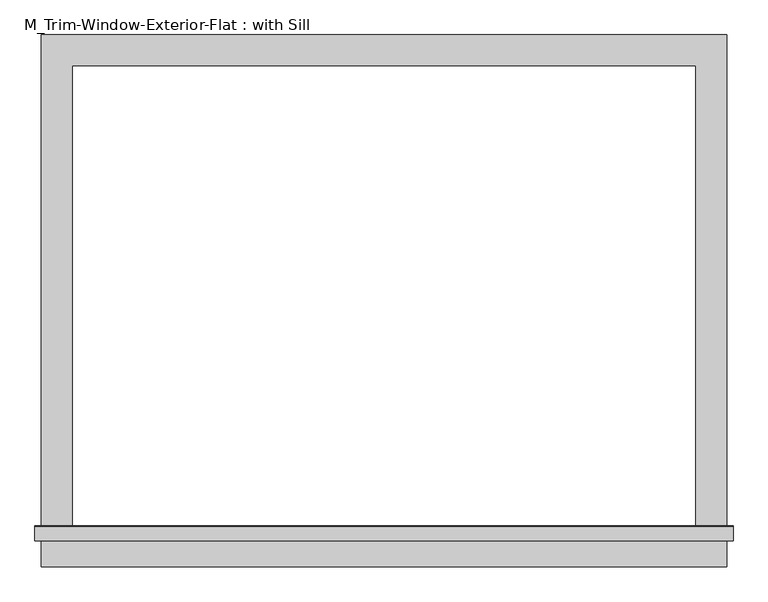
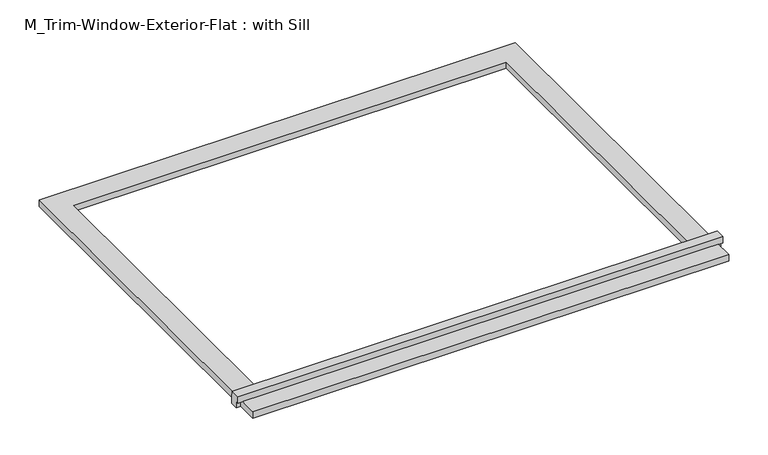
"""IFC4 building model written with IfcOpenShell, lengths in millimetres: proxy geometry, M_Trim-Window-Exterior-Flat : with Sill."""

from ifc_helpers import new_model, si_unit, frame, origin, origin_with_axes, place, context, project, spatial, polyline, outline, extrude, source, transform, mapped, element, save


def m_trim_window_exterior_flat_with_sill_b1b88069(model_context):
    return source(origin(), model_context, "Body", "SweptSolid", [
        extrude(outline(polyline([(669.6, -920.4323709), (669.6, -980.4323709), (-669.6, -980.4323709), (-669.6, -920.4323709), (669.6, -920.4323709)])), origin_with_axes(), (0.0, 0.0, 1.0), 19.05),
        extrude(outline(polyline([(-930.0, 38.1), (-902.4580645, 38.1), (-900.0, 19.05), (-900.0, 0.0), (-920.4323709, 0.0), (-920.4323709, 19.05), (-930.0, 19.05), (-930.0, 38.1)])), frame((-682.3, 0.0, 0.0), z_axis=(1.0, 0.0, 0.0), x_axis=(0.0, 1.0, 0.0)), (0.0, 0.0, 1.0), 1364.6),
        extrude(outline(polyline([(-669.6, 60.0), (669.6, 60.0), (669.6, -900.0), (609.6, -900.0), (609.6, 0.0), (-609.6, 0.0), (-609.6, -900.0), (-669.6, -900.0), (-669.6, 60.0)])), origin_with_axes(), (0.0, 0.0, 1.0), 19.05),
    ])


if __name__ == "__main__":
    model = new_model("IFC4")
    model_context = context("Model", 3, world=origin())
    ifc_project = project(units=[si_unit("LENGTHUNIT", "METRE", prefix="MILLI")], contexts=[model_context])
    site = spatial("IfcSite", under=ifc_project)
    building = spatial("IfcBuilding", under=site)
    placement = place(None, origin())
    m_trim_window_exterior_flat_with_sill_shape = m_trim_window_exterior_flat_with_sill_b1b88069(model_context)
    element("IfcBuildingElementProxy", 1, Name="M_Trim-Window-Exterior-Flat : with Sill", ObjectType="M_Trim-Window-Exterior-Flat : with Sill", at=placement, inside=building, context=model_context, shape_type="MappedRepresentation", body=[
        mapped(m_trim_window_exterior_flat_with_sill_shape, transform((0.0, 0.0, 0.0), x_axis=(1.0, 0.0, 0.0), y_axis=(0.0, 1.0, 0.0), z_axis=(0.0, 0.0, 1.0))),
    ])
    save(model, "model.ifc")

# Revit data of these elements
# Type "M_Trim-Window-Exterior-Flat : with Sill"
#   Trim Width = 0' - 2.3622"
#   Trim Thickness_Picture Frame = 0' - 1.1811"
#   Trim Thickness_with Sill = 0' - 0 3/4"
#   Sill Thickness = 0' - 1.1811"
#   Opening Width [instance default] = 1' - 11.62205"
#   Opening Height [instance default] = 2' - 11.43307"
#   Default Elevation = 3' - 11.24409"
#   Sill = yes
#   Picture Frame = no
#   Trim Material [instance default] = none
# Element 1 (IfcBuildingElementProxy, "M_Trim-Window-Exterior-Flat : with Sill")
#   Opening Width = 4' - 0"
#   Trim Material = Clad - White
#   Materials on its faces: "Clad - White"
# Materials
#   "Clad - White": class "Wood", colour RGB 242 242 238, transparency 0, Cost = 0
